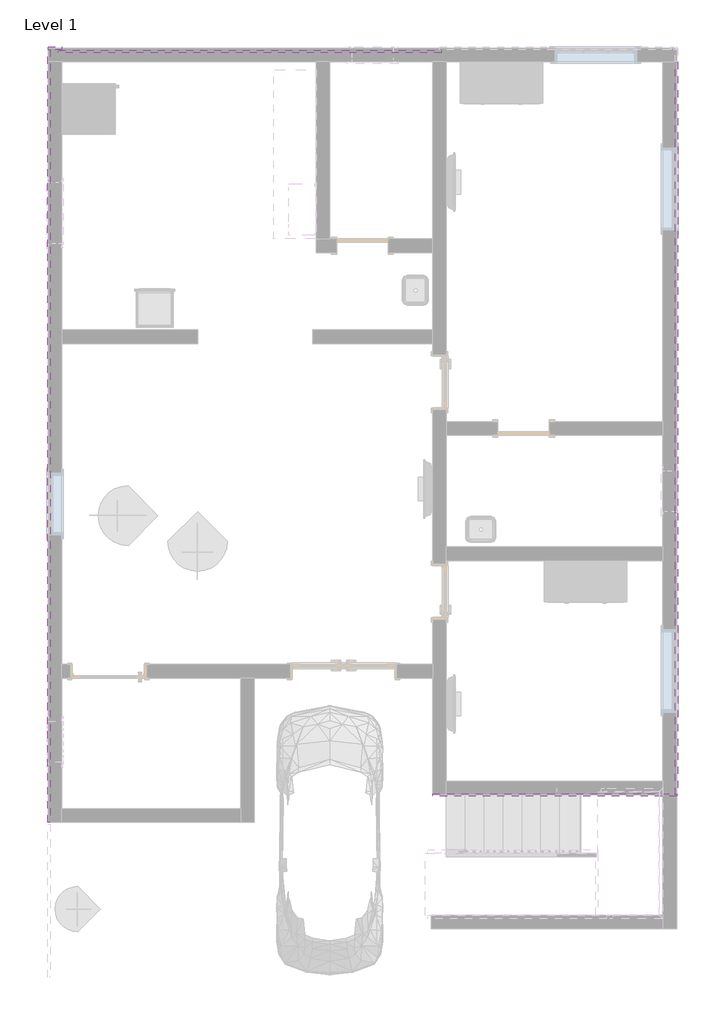
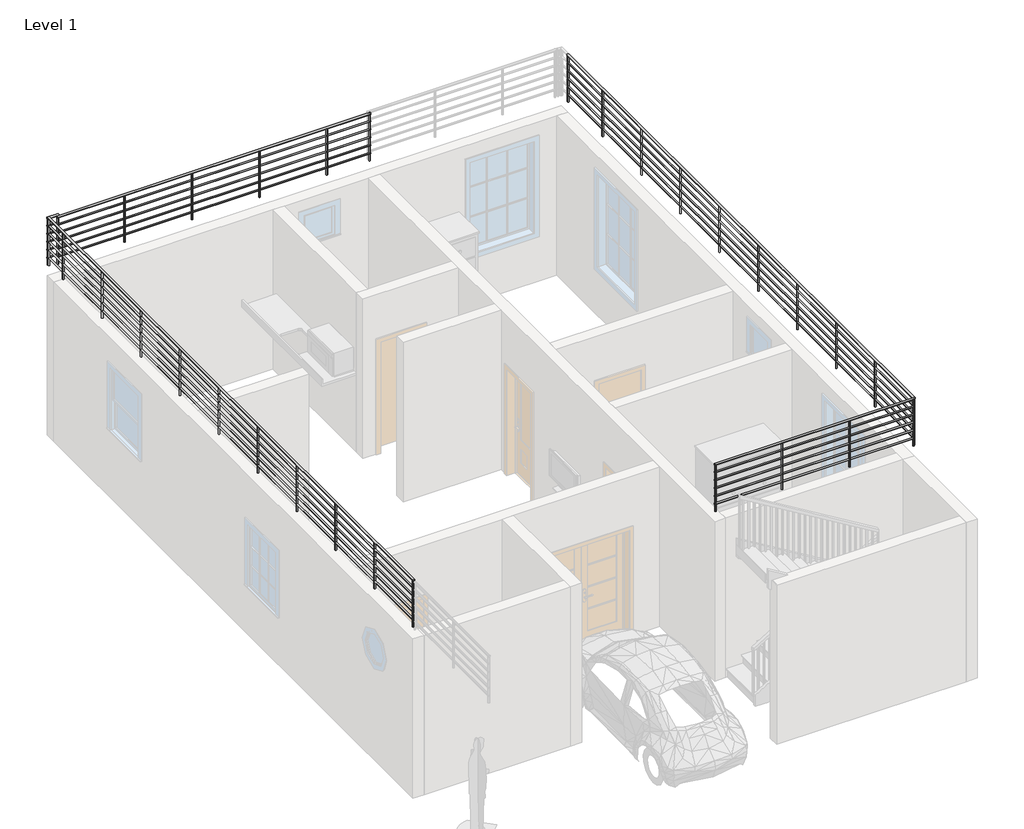
# One storey, part 3 of 4: 5 railings.
"""IFC4 building model written with IfcOpenShell, lengths in millimetres."""

from ifc_helpers import new_model, si_unit, point, frame, frame_2d, origin, place, context, project, spatial, circle_curve, trimmed, segment, composite_curve, outline, extrude, element, save

model = new_model("IFC4")

# Units and contexts
model_context = context("Model", 3, world=origin())
ifc_project = project(units=[si_unit("LENGTHUNIT", "METRE", prefix="MILLI")], contexts=[model_context])

# Site, building, storey
site = spatial("IfcSite", under=ifc_project)
building = spatial("IfcBuilding", under=site)
storey = spatial("IfcBuildingStorey", under=building, Name="Level 1", Elevation=0.0)

# Railings
placement = place(None, origin())
element("IfcRailing", 1, ObjectType="Handrail - Pipe", at=placement, inside=storey, context=model_context, shape_type="SweptSolid", body=[
    extrude(outline(composite_curve([segment(trimmed(circle_curve(frame_2d((4165.6002567, -14409.9389568)), 19.05), [point((4165.6002567, -14390.8889568))], [point((4165.6002567, -14428.9889568))], False, "CARTESIAN"), True, "CONTINUOUS"), segment(trimmed(circle_curve(frame_2d((4165.6002567, -14409.9389568)), 19.05), [point((4165.6002567, -14428.9889568))], [point((4165.6002567, -14390.8889568))], False, "CARTESIAN"), True, "CONTINUOUS")], self_intersect=False)), frame((0.0, 3652.9401605, 0.0), z_axis=(0.0, 1.0, 0.0), x_axis=(0.0, 0.0, 1.0)), (0.0, 0.0, 1.0), 11430.0),
    extrude(outline(composite_curve([segment(trimmed(circle_curve(frame_2d((4019.5502567, -14409.9389568)), 12.7), [point((4019.5502567, -14422.6389568))], [point((4019.5502567, -14397.2389568))], False, "CARTESIAN"), True, "CONTINUOUS"), segment(trimmed(circle_curve(frame_2d((4019.5502567, -14409.9389568)), 12.7), [point((4019.5502567, -14397.2389568))], [point((4019.5502567, -14422.6389568))], False, "CARTESIAN"), True, "CONTINUOUS")], self_intersect=False)), frame((0.0, 3652.9401605, 0.0), z_axis=(0.0, 1.0, 0.0), x_axis=(0.0, 0.0, 1.0)), (0.0, 0.0, 1.0), 11430.0),
    extrude(outline(composite_curve([segment(trimmed(circle_curve(frame_2d((3867.1502567, -14409.9389568)), 12.7), [point((3867.1502567, -14422.6389568))], [point((3867.1502567, -14397.2389568))], False, "CARTESIAN"), True, "CONTINUOUS"), segment(trimmed(circle_curve(frame_2d((3867.1502567, -14409.9389568)), 12.7), [point((3867.1502567, -14397.2389568))], [point((3867.1502567, -14422.6389568))], False, "CARTESIAN"), True, "CONTINUOUS")], self_intersect=False)), frame((0.0, 3652.9401605, 0.0), z_axis=(0.0, 1.0, 0.0), x_axis=(0.0, 0.0, 1.0)), (0.0, 0.0, 1.0), 11430.0),
    extrude(outline(composite_curve([segment(trimmed(circle_curve(frame_2d((3714.7502567, -14409.9389568)), 12.7), [point((3714.7502567, -14422.6389568))], [point((3714.7502567, -14397.2389568))], False, "CARTESIAN"), True, "CONTINUOUS"), segment(trimmed(circle_curve(frame_2d((3714.7502567, -14409.9389568)), 12.7), [point((3714.7502567, -14397.2389568))], [point((3714.7502567, -14422.6389568))], False, "CARTESIAN"), True, "CONTINUOUS")], self_intersect=False)), frame((0.0, 3652.9401605, 0.0), z_axis=(0.0, 1.0, 0.0), x_axis=(0.0, 0.0, 1.0)), (0.0, 0.0, 1.0), 11430.0),
    extrude(outline(composite_curve([segment(trimmed(circle_curve(frame_2d((3562.3502567, -14409.9389568)), 12.7), [point((3562.3502567, -14422.6389568))], [point((3562.3502567, -14397.2389568))], False, "CARTESIAN"), True, "CONTINUOUS"), segment(trimmed(circle_curve(frame_2d((3562.3502567, -14409.9389568)), 12.7), [point((3562.3502567, -14397.2389568))], [point((3562.3502567, -14422.6389568))], False, "CARTESIAN"), True, "CONTINUOUS")], self_intersect=False)), frame((0.0, 3652.9401605, 0.0), z_axis=(0.0, 1.0, 0.0), x_axis=(0.0, 0.0, 1.0)), (0.0, 0.0, 1.0), 11430.0),
    extrude(outline(composite_curve([segment(trimmed(circle_curve(frame_2d((3409.9502567, -14409.9389568)), 12.7), [point((3409.9502567, -14422.6389568))], [point((3409.9502567, -14397.2389568))], False, "CARTESIAN"), True, "CONTINUOUS"), segment(trimmed(circle_curve(frame_2d((3409.9502567, -14409.9389568)), 12.7), [point((3409.9502567, -14397.2389568))], [point((3409.9502567, -14422.6389568))], False, "CARTESIAN"), True, "CONTINUOUS")], self_intersect=False)), frame((0.0, 3652.9401605, 0.0), z_axis=(0.0, 1.0, 0.0), x_axis=(0.0, 0.0, 1.0)), (0.0, 0.0, 1.0), 11430.0),
    extrude(outline(composite_curve([segment(trimmed(circle_curve(frame_2d((-14409.9389568, 14625.7401605)), 12.7), [point((-14422.6389568, 14625.7401605))], [point((-14397.2389568, 14625.7401605))], False, "CARTESIAN"), True, "CONTINUOUS"), segment(trimmed(circle_curve(frame_2d((-14409.9389568, 14625.7401605)), 12.7), [point((-14397.2389568, 14625.7401605))], [point((-14422.6389568, 14625.7401605))], False, "CARTESIAN"), True, "CONTINUOUS")], self_intersect=False)), frame((0.0, 0.0, 3270.2502567), z_axis=(0.0, 0.0, 1.0), x_axis=(1.0, 0.0, 0.0)), (0.0, 0.0, 1.0), 876.3),
    extrude(outline(composite_curve([segment(trimmed(circle_curve(frame_2d((-14409.9389568, 13406.5401605)), 12.7), [point((-14422.6389568, 13406.5401605))], [point((-14397.2389568, 13406.5401605))], False, "CARTESIAN"), True, "CONTINUOUS"), segment(trimmed(circle_curve(frame_2d((-14409.9389568, 13406.5401605)), 12.7), [point((-14397.2389568, 13406.5401605))], [point((-14422.6389568, 13406.5401605))], False, "CARTESIAN"), True, "CONTINUOUS")], self_intersect=False)), frame((0.0, 0.0, 3270.2502567), z_axis=(0.0, 0.0, 1.0), x_axis=(1.0, 0.0, 0.0)), (0.0, 0.0, 1.0), 876.3),
    extrude(outline(composite_curve([segment(trimmed(circle_curve(frame_2d((-14409.9389568, 12187.3401605)), 12.7), [point((-14422.6389568, 12187.3401605))], [point((-14397.2389568, 12187.3401605))], False, "CARTESIAN"), True, "CONTINUOUS"), segment(trimmed(circle_curve(frame_2d((-14409.9389568, 12187.3401605)), 12.7), [point((-14397.2389568, 12187.3401605))], [point((-14422.6389568, 12187.3401605))], False, "CARTESIAN"), True, "CONTINUOUS")], self_intersect=False)), frame((0.0, 0.0, 3270.2502567), z_axis=(0.0, 0.0, 1.0), x_axis=(1.0, 0.0, 0.0)), (0.0, 0.0, 1.0), 876.3),
    extrude(outline(composite_curve([segment(trimmed(circle_curve(frame_2d((-14409.9389568, 10968.1401605)), 12.7), [point((-14422.6389568, 10968.1401605))], [point((-14397.2389568, 10968.1401605))], False, "CARTESIAN"), True, "CONTINUOUS"), segment(trimmed(circle_curve(frame_2d((-14409.9389568, 10968.1401605)), 12.7), [point((-14397.2389568, 10968.1401605))], [point((-14422.6389568, 10968.1401605))], False, "CARTESIAN"), True, "CONTINUOUS")], self_intersect=False)), frame((0.0, 0.0, 3270.2502567), z_axis=(0.0, 0.0, 1.0), x_axis=(1.0, 0.0, 0.0)), (0.0, 0.0, 1.0), 876.3),
    extrude(outline(composite_curve([segment(trimmed(circle_curve(frame_2d((-14409.9389568, 9748.9401605)), 12.7), [point((-14422.6389568, 9748.9401605))], [point((-14397.2389568, 9748.9401605))], False, "CARTESIAN"), True, "CONTINUOUS"), segment(trimmed(circle_curve(frame_2d((-14409.9389568, 9748.9401605)), 12.7), [point((-14397.2389568, 9748.9401605))], [point((-14422.6389568, 9748.9401605))], False, "CARTESIAN"), True, "CONTINUOUS")], self_intersect=False)), frame((0.0, 0.0, 3270.2502567), z_axis=(0.0, 0.0, 1.0), x_axis=(1.0, 0.0, 0.0)), (0.0, 0.0, 1.0), 876.3),
    extrude(outline(composite_curve([segment(trimmed(circle_curve(frame_2d((-14409.9389568, 8529.7401605)), 12.7), [point((-14422.6389568, 8529.7401605))], [point((-14397.2389568, 8529.7401605))], False, "CARTESIAN"), True, "CONTINUOUS"), segment(trimmed(circle_curve(frame_2d((-14409.9389568, 8529.7401605)), 12.7), [point((-14397.2389568, 8529.7401605))], [point((-14422.6389568, 8529.7401605))], False, "CARTESIAN"), True, "CONTINUOUS")], self_intersect=False)), frame((0.0, 0.0, 3270.2502567), z_axis=(0.0, 0.0, 1.0), x_axis=(1.0, 0.0, 0.0)), (0.0, 0.0, 1.0), 876.3),
    extrude(outline(composite_curve([segment(trimmed(circle_curve(frame_2d((-14409.9389568, 7310.5401605)), 12.7), [point((-14422.6389568, 7310.5401605))], [point((-14397.2389568, 7310.5401605))], False, "CARTESIAN"), True, "CONTINUOUS"), segment(trimmed(circle_curve(frame_2d((-14409.9389568, 7310.5401605)), 12.7), [point((-14397.2389568, 7310.5401605))], [point((-14422.6389568, 7310.5401605))], False, "CARTESIAN"), True, "CONTINUOUS")], self_intersect=False)), frame((0.0, 0.0, 3270.2502567), z_axis=(0.0, 0.0, 1.0), x_axis=(1.0, 0.0, 0.0)), (0.0, 0.0, 1.0), 876.3),
    extrude(outline(composite_curve([segment(trimmed(circle_curve(frame_2d((-14409.9389568, 6091.3401605)), 12.7), [point((-14422.6389568, 6091.3401605))], [point((-14397.2389568, 6091.3401605))], False, "CARTESIAN"), True, "CONTINUOUS"), segment(trimmed(circle_curve(frame_2d((-14409.9389568, 6091.3401605)), 12.7), [point((-14397.2389568, 6091.3401605))], [point((-14422.6389568, 6091.3401605))], False, "CARTESIAN"), True, "CONTINUOUS")], self_intersect=False)), frame((0.0, 0.0, 3270.2502567), z_axis=(0.0, 0.0, 1.0), x_axis=(1.0, 0.0, 0.0)), (0.0, 0.0, 1.0), 876.3),
    extrude(outline(composite_curve([segment(trimmed(circle_curve(frame_2d((-14409.9389568, 4872.1401605)), 12.7), [point((-14422.6389568, 4872.1401605))], [point((-14397.2389568, 4872.1401605))], False, "CARTESIAN"), True, "CONTINUOUS"), segment(trimmed(circle_curve(frame_2d((-14409.9389568, 4872.1401605)), 12.7), [point((-14397.2389568, 4872.1401605))], [point((-14422.6389568, 4872.1401605))], False, "CARTESIAN"), True, "CONTINUOUS")], self_intersect=False)), frame((0.0, 0.0, 3270.2502567), z_axis=(0.0, 0.0, 1.0), x_axis=(1.0, 0.0, 0.0)), (0.0, 0.0, 1.0), 876.3),
    extrude(outline(composite_curve([segment(trimmed(circle_curve(frame_2d((-14409.9389568, 15070.2401605)), 12.7), [point((-14422.6389568, 15070.2401605))], [point((-14397.2389568, 15070.2401605))], False, "CARTESIAN"), True, "CONTINUOUS"), segment(trimmed(circle_curve(frame_2d((-14409.9389568, 15070.2401605)), 12.7), [point((-14397.2389568, 15070.2401605))], [point((-14422.6389568, 15070.2401605))], False, "CARTESIAN"), True, "CONTINUOUS")], self_intersect=False)), frame((0.0, 0.0, 3270.2502567), z_axis=(0.0, 0.0, 1.0), x_axis=(1.0, 0.0, 0.0)), (0.0, 0.0, 1.0), 876.3),
    extrude(outline(composite_curve([segment(trimmed(circle_curve(frame_2d((-14409.9389568, 3665.6401605)), 12.7), [point((-14422.6389568, 3665.6401605))], [point((-14397.2389568, 3665.6401605))], False, "CARTESIAN"), True, "CONTINUOUS"), segment(trimmed(circle_curve(frame_2d((-14409.9389568, 3665.6401605)), 12.7), [point((-14397.2389568, 3665.6401605))], [point((-14422.6389568, 3665.6401605))], False, "CARTESIAN"), True, "CONTINUOUS")], self_intersect=False)), frame((0.0, 0.0, 3270.2502567), z_axis=(0.0, 0.0, 1.0), x_axis=(1.0, 0.0, 0.0)), (0.0, 0.0, 1.0), 876.3),
])
element("IfcRailing", 2, ObjectType="Handrail - Pipe", at=placement, inside=storey, context=model_context, shape_type="SweptSolid", body=[
    extrude(outline(composite_curve([segment(trimmed(circle_curve(frame_2d((15057.9844698, 4146.55)), 19.05), [point((15038.9344698, 4146.55))], [point((15077.0344698, 4146.55))], False, "CARTESIAN"), True, "CONTINUOUS"), segment(trimmed(circle_curve(frame_2d((15057.9844698, 4146.55)), 19.05), [point((15077.0344698, 4146.55))], [point((15038.9344698, 4146.55))], False, "CARTESIAN"), True, "CONTINUOUS")], self_intersect=False)), frame((-14272.3568408, 0.0, 0.0), z_axis=(1.0, 0.0, 0.0), x_axis=(0.0, 1.0, 0.0)), (0.0, 0.0, 1.0), 5664.2),
    extrude(outline(composite_curve([segment(trimmed(circle_curve(frame_2d((15057.9844698, 4000.5)), 12.7), [point((15070.6844698, 4000.5))], [point((15045.2844698, 4000.5))], False, "CARTESIAN"), True, "CONTINUOUS"), segment(trimmed(circle_curve(frame_2d((15057.9844698, 4000.5)), 12.7), [point((15045.2844698, 4000.5))], [point((15070.6844698, 4000.5))], False, "CARTESIAN"), True, "CONTINUOUS")], self_intersect=False)), frame((-14272.3568408, 0.0, 0.0), z_axis=(1.0, 0.0, 0.0), x_axis=(0.0, 1.0, 0.0)), (0.0, 0.0, 1.0), 5664.2),
    extrude(outline(composite_curve([segment(trimmed(circle_curve(frame_2d((15057.9844698, 3848.1)), 12.7), [point((15070.6844698, 3848.1))], [point((15045.2844698, 3848.1))], False, "CARTESIAN"), True, "CONTINUOUS"), segment(trimmed(circle_curve(frame_2d((15057.9844698, 3848.1)), 12.7), [point((15045.2844698, 3848.1))], [point((15070.6844698, 3848.1))], False, "CARTESIAN"), True, "CONTINUOUS")], self_intersect=False)), frame((-14272.3568408, 0.0, 0.0), z_axis=(1.0, 0.0, 0.0), x_axis=(0.0, 1.0, 0.0)), (0.0, 0.0, 1.0), 5664.2),
    extrude(outline(composite_curve([segment(trimmed(circle_curve(frame_2d((15057.9844698, 3695.7)), 12.7), [point((15070.6844698, 3695.7))], [point((15045.2844698, 3695.7))], False, "CARTESIAN"), True, "CONTINUOUS"), segment(trimmed(circle_curve(frame_2d((15057.9844698, 3695.7)), 12.7), [point((15045.2844698, 3695.7))], [point((15070.6844698, 3695.7))], False, "CARTESIAN"), True, "CONTINUOUS")], self_intersect=False)), frame((-14272.3568408, 0.0, 0.0), z_axis=(1.0, 0.0, 0.0), x_axis=(0.0, 1.0, 0.0)), (0.0, 0.0, 1.0), 5664.2),
    extrude(outline(composite_curve([segment(trimmed(circle_curve(frame_2d((15057.9844698, 3543.3)), 12.7), [point((15070.6844698, 3543.3))], [point((15045.2844698, 3543.3))], False, "CARTESIAN"), True, "CONTINUOUS"), segment(trimmed(circle_curve(frame_2d((15057.9844698, 3543.3)), 12.7), [point((15045.2844698, 3543.3))], [point((15070.6844698, 3543.3))], False, "CARTESIAN"), True, "CONTINUOUS")], self_intersect=False)), frame((-14272.3568408, 0.0, 0.0), z_axis=(1.0, 0.0, 0.0), x_axis=(0.0, 1.0, 0.0)), (0.0, 0.0, 1.0), 5664.2),
    extrude(outline(composite_curve([segment(trimmed(circle_curve(frame_2d((15057.9844698, 3390.9)), 12.7), [point((15070.6844698, 3390.9))], [point((15045.2844698, 3390.9))], False, "CARTESIAN"), True, "CONTINUOUS"), segment(trimmed(circle_curve(frame_2d((15057.9844698, 3390.9)), 12.7), [point((15045.2844698, 3390.9))], [point((15070.6844698, 3390.9))], False, "CARTESIAN"), True, "CONTINUOUS")], self_intersect=False)), frame((-14272.3568408, 0.0, 0.0), z_axis=(1.0, 0.0, 0.0), x_axis=(0.0, 1.0, 0.0)), (0.0, 0.0, 1.0), 5664.2),
    extrude(outline(composite_curve([segment(trimmed(circle_curve(frame_2d((-9395.5568408, 15057.9844698)), 12.7), [point((-9395.5568408, 15070.6844698))], [point((-9395.5568408, 15045.2844698))], False, "CARTESIAN"), True, "CONTINUOUS"), segment(trimmed(circle_curve(frame_2d((-9395.5568408, 15057.9844698)), 12.7), [point((-9395.5568408, 15045.2844698))], [point((-9395.5568408, 15070.6844698))], False, "CARTESIAN"), True, "CONTINUOUS")], self_intersect=False)), frame((0.0, 0.0, 3251.2), z_axis=(0.0, 0.0, 1.0), x_axis=(1.0, 0.0, 0.0)), (0.0, 0.0, 1.0), 876.3),
    extrude(outline(composite_curve([segment(trimmed(circle_curve(frame_2d((-10614.7568408, 15057.9844698)), 12.7), [point((-10614.7568408, 15070.6844698))], [point((-10614.7568408, 15045.2844698))], False, "CARTESIAN"), True, "CONTINUOUS"), segment(trimmed(circle_curve(frame_2d((-10614.7568408, 15057.9844698)), 12.7), [point((-10614.7568408, 15045.2844698))], [point((-10614.7568408, 15070.6844698))], False, "CARTESIAN"), True, "CONTINUOUS")], self_intersect=False)), frame((0.0, 0.0, 3251.2), z_axis=(0.0, 0.0, 1.0), x_axis=(1.0, 0.0, 0.0)), (0.0, 0.0, 1.0), 876.3),
    extrude(outline(composite_curve([segment(trimmed(circle_curve(frame_2d((-11833.9568408, 15057.9844698)), 12.7), [point((-11833.9568408, 15070.6844698))], [point((-11833.9568408, 15045.2844698))], False, "CARTESIAN"), True, "CONTINUOUS"), segment(trimmed(circle_curve(frame_2d((-11833.9568408, 15057.9844698)), 12.7), [point((-11833.9568408, 15045.2844698))], [point((-11833.9568408, 15070.6844698))], False, "CARTESIAN"), True, "CONTINUOUS")], self_intersect=False)), frame((0.0, 0.0, 3251.2), z_axis=(0.0, 0.0, 1.0), x_axis=(1.0, 0.0, 0.0)), (0.0, 0.0, 1.0), 876.3),
    extrude(outline(composite_curve([segment(trimmed(circle_curve(frame_2d((-13053.1568408, 15057.9844698)), 12.7), [point((-13053.1568408, 15070.6844698))], [point((-13053.1568408, 15045.2844698))], False, "CARTESIAN"), True, "CONTINUOUS"), segment(trimmed(circle_curve(frame_2d((-13053.1568408, 15057.9844698)), 12.7), [point((-13053.1568408, 15045.2844698))], [point((-13053.1568408, 15070.6844698))], False, "CARTESIAN"), True, "CONTINUOUS")], self_intersect=False)), frame((0.0, 0.0, 3251.2), z_axis=(0.0, 0.0, 1.0), x_axis=(1.0, 0.0, 0.0)), (0.0, 0.0, 1.0), 876.3),
    extrude(outline(composite_curve([segment(trimmed(circle_curve(frame_2d((-8620.8568408, 15057.9844698)), 12.7), [point((-8620.8568408, 15070.6844698))], [point((-8620.8568408, 15045.2844698))], False, "CARTESIAN"), True, "CONTINUOUS"), segment(trimmed(circle_curve(frame_2d((-8620.8568408, 15057.9844698)), 12.7), [point((-8620.8568408, 15045.2844698))], [point((-8620.8568408, 15070.6844698))], False, "CARTESIAN"), True, "CONTINUOUS")], self_intersect=False)), frame((0.0, 0.0, 3251.2), z_axis=(0.0, 0.0, 1.0), x_axis=(1.0, 0.0, 0.0)), (0.0, 0.0, 1.0), 876.3),
    extrude(outline(composite_curve([segment(trimmed(circle_curve(frame_2d((-14259.6568408, 15057.9844698)), 12.7), [point((-14259.6568408, 15070.6844698))], [point((-14259.6568408, 15045.2844698))], False, "CARTESIAN"), True, "CONTINUOUS"), segment(trimmed(circle_curve(frame_2d((-14259.6568408, 15057.9844698)), 12.7), [point((-14259.6568408, 15045.2844698))], [point((-14259.6568408, 15070.6844698))], False, "CARTESIAN"), True, "CONTINUOUS")], self_intersect=False)), frame((0.0, 0.0, 3251.2), z_axis=(0.0, 0.0, 1.0), x_axis=(1.0, 0.0, 0.0)), (0.0, 0.0, 1.0), 876.3),
])
element("IfcRailing", 3, ObjectType="Handrail - Pipe", at=placement, inside=storey, context=model_context, shape_type="SweptSolid", body=[
    extrude(outline(composite_curve([segment(trimmed(circle_curve(frame_2d((4059.1342758, 4146.55)), 19.05), [point((4040.0842758, 4146.55))], [point((4078.1842758, 4146.55))], False, "CARTESIAN"), True, "CONTINUOUS"), segment(trimmed(circle_curve(frame_2d((4059.1342758, 4146.55)), 19.05), [point((4078.1842758, 4146.55))], [point((4040.0842758, 4146.55))], False, "CARTESIAN"), True, "CONTINUOUS")], self_intersect=False)), frame((-8733.0389568, 0.0, 0.0), z_axis=(1.0, 0.0, 0.0), x_axis=(0.0, 1.0, 0.0)), (0.0, 0.0, 1.0), 3606.8),
    extrude(outline(composite_curve([segment(trimmed(circle_curve(frame_2d((4059.1342758, 4000.5)), 12.7), [point((4071.8342758, 4000.5))], [point((4046.4342758, 4000.5))], False, "CARTESIAN"), True, "CONTINUOUS"), segment(trimmed(circle_curve(frame_2d((4059.1342758, 4000.5)), 12.7), [point((4046.4342758, 4000.5))], [point((4071.8342758, 4000.5))], False, "CARTESIAN"), True, "CONTINUOUS")], self_intersect=False)), frame((-8733.0389568, 0.0, 0.0), z_axis=(1.0, 0.0, 0.0), x_axis=(0.0, 1.0, 0.0)), (0.0, 0.0, 1.0), 3606.8),
    extrude(outline(composite_curve([segment(trimmed(circle_curve(frame_2d((4059.1342758, 3848.1)), 12.7), [point((4071.8342758, 3848.1))], [point((4046.4342758, 3848.1))], False, "CARTESIAN"), True, "CONTINUOUS"), segment(trimmed(circle_curve(frame_2d((4059.1342758, 3848.1)), 12.7), [point((4046.4342758, 3848.1))], [point((4071.8342758, 3848.1))], False, "CARTESIAN"), True, "CONTINUOUS")], self_intersect=False)), frame((-8733.0389568, 0.0, 0.0), z_axis=(1.0, 0.0, 0.0), x_axis=(0.0, 1.0, 0.0)), (0.0, 0.0, 1.0), 3606.8),
    extrude(outline(composite_curve([segment(trimmed(circle_curve(frame_2d((4059.1342758, 3695.7)), 12.7), [point((4071.8342758, 3695.7))], [point((4046.4342758, 3695.7))], False, "CARTESIAN"), True, "CONTINUOUS"), segment(trimmed(circle_curve(frame_2d((4059.1342758, 3695.7)), 12.7), [point((4046.4342758, 3695.7))], [point((4071.8342758, 3695.7))], False, "CARTESIAN"), True, "CONTINUOUS")], self_intersect=False)), frame((-8733.0389568, 0.0, 0.0), z_axis=(1.0, 0.0, 0.0), x_axis=(0.0, 1.0, 0.0)), (0.0, 0.0, 1.0), 3606.8),
    extrude(outline(composite_curve([segment(trimmed(circle_curve(frame_2d((4059.1342758, 3543.3)), 12.7), [point((4071.8342758, 3543.3))], [point((4046.4342758, 3543.3))], False, "CARTESIAN"), True, "CONTINUOUS"), segment(trimmed(circle_curve(frame_2d((4059.1342758, 3543.3)), 12.7), [point((4046.4342758, 3543.3))], [point((4071.8342758, 3543.3))], False, "CARTESIAN"), True, "CONTINUOUS")], self_intersect=False)), frame((-8733.0389568, 0.0, 0.0), z_axis=(1.0, 0.0, 0.0), x_axis=(0.0, 1.0, 0.0)), (0.0, 0.0, 1.0), 3606.8),
    extrude(outline(composite_curve([segment(trimmed(circle_curve(frame_2d((4059.1342758, 3390.9)), 12.7), [point((4071.8342758, 3390.9))], [point((4046.4342758, 3390.9))], False, "CARTESIAN"), True, "CONTINUOUS"), segment(trimmed(circle_curve(frame_2d((4059.1342758, 3390.9)), 12.7), [point((4046.4342758, 3390.9))], [point((4071.8342758, 3390.9))], False, "CARTESIAN"), True, "CONTINUOUS")], self_intersect=False)), frame((-8733.0389568, 0.0, 0.0), z_axis=(1.0, 0.0, 0.0), x_axis=(0.0, 1.0, 0.0)), (0.0, 0.0, 1.0), 3606.8),
    extrude(outline(composite_curve([segment(trimmed(circle_curve(frame_2d((-6294.6389568, 4059.1342758)), 12.7), [point((-6294.6389568, 4071.8342758))], [point((-6294.6389568, 4046.4342758))], False, "CARTESIAN"), True, "CONTINUOUS"), segment(trimmed(circle_curve(frame_2d((-6294.6389568, 4059.1342758)), 12.7), [point((-6294.6389568, 4046.4342758))], [point((-6294.6389568, 4071.8342758))], False, "CARTESIAN"), True, "CONTINUOUS")], self_intersect=False)), frame((0.0, 0.0, 3251.2), z_axis=(0.0, 0.0, 1.0), x_axis=(1.0, 0.0, 0.0)), (0.0, 0.0, 1.0), 876.3),
    extrude(outline(composite_curve([segment(trimmed(circle_curve(frame_2d((-7513.8389568, 4059.1342758)), 12.7), [point((-7513.8389568, 4071.8342758))], [point((-7513.8389568, 4046.4342758))], False, "CARTESIAN"), True, "CONTINUOUS"), segment(trimmed(circle_curve(frame_2d((-7513.8389568, 4059.1342758)), 12.7), [point((-7513.8389568, 4046.4342758))], [point((-7513.8389568, 4071.8342758))], False, "CARTESIAN"), True, "CONTINUOUS")], self_intersect=False)), frame((0.0, 0.0, 3251.2), z_axis=(0.0, 0.0, 1.0), x_axis=(1.0, 0.0, 0.0)), (0.0, 0.0, 1.0), 876.3),
    extrude(outline(composite_curve([segment(trimmed(circle_curve(frame_2d((-5138.9389568, 4059.1342758)), 12.7), [point((-5138.9389568, 4071.8342758))], [point((-5138.9389568, 4046.4342758))], False, "CARTESIAN"), True, "CONTINUOUS"), segment(trimmed(circle_curve(frame_2d((-5138.9389568, 4059.1342758)), 12.7), [point((-5138.9389568, 4046.4342758))], [point((-5138.9389568, 4071.8342758))], False, "CARTESIAN"), True, "CONTINUOUS")], self_intersect=False)), frame((0.0, 0.0, 3251.2), z_axis=(0.0, 0.0, 1.0), x_axis=(1.0, 0.0, 0.0)), (0.0, 0.0, 1.0), 876.3),
    extrude(outline(composite_curve([segment(trimmed(circle_curve(frame_2d((-8720.3389568, 4059.1342758)), 12.7), [point((-8720.3389568, 4071.8342758))], [point((-8720.3389568, 4046.4342758))], False, "CARTESIAN"), True, "CONTINUOUS"), segment(trimmed(circle_curve(frame_2d((-8720.3389568, 4059.1342758)), 12.7), [point((-8720.3389568, 4046.4342758))], [point((-8720.3389568, 4071.8342758))], False, "CARTESIAN"), True, "CONTINUOUS")], self_intersect=False)), frame((0.0, 0.0, 3251.2), z_axis=(0.0, 0.0, 1.0), x_axis=(1.0, 0.0, 0.0)), (0.0, 0.0, 1.0), 876.3),
])
element("IfcRailing", 4, ObjectType="Handrail - Pipe", at=placement, inside=storey, context=model_context, shape_type="SweptSolid", body=[
    extrude(outline(composite_curve([segment(trimmed(circle_curve(frame_2d((4146.55, -5126.2389568)), 19.05), [point((4146.55, -5107.1889568))], [point((4146.55, -5145.2889568))], False, "CARTESIAN"), True, "CONTINUOUS"), segment(trimmed(circle_curve(frame_2d((4146.55, -5126.2389568)), 19.05), [point((4146.55, -5145.2889568))], [point((4146.55, -5107.1889568))], False, "CARTESIAN"), True, "CONTINUOUS")], self_intersect=False)), frame((0.0, 4059.1342758, 0.0), z_axis=(0.0, 1.0, 0.0), x_axis=(0.0, 0.0, 1.0)), (0.0, 0.0, 1.0), 10845.8),
    extrude(outline(composite_curve([segment(trimmed(circle_curve(frame_2d((4000.5, -5126.2389568)), 12.7), [point((4000.5, -5138.9389568))], [point((4000.5, -5113.5389568))], False, "CARTESIAN"), True, "CONTINUOUS"), segment(trimmed(circle_curve(frame_2d((4000.5, -5126.2389568)), 12.7), [point((4000.5, -5113.5389568))], [point((4000.5, -5138.9389568))], False, "CARTESIAN"), True, "CONTINUOUS")], self_intersect=False)), frame((0.0, 4059.1342758, 0.0), z_axis=(0.0, 1.0, 0.0), x_axis=(0.0, 0.0, 1.0)), (0.0, 0.0, 1.0), 10845.8),
    extrude(outline(composite_curve([segment(trimmed(circle_curve(frame_2d((3848.1, -5126.2389568)), 12.7), [point((3848.1, -5138.9389568))], [point((3848.1, -5113.5389568))], False, "CARTESIAN"), True, "CONTINUOUS"), segment(trimmed(circle_curve(frame_2d((3848.1, -5126.2389568)), 12.7), [point((3848.1, -5113.5389568))], [point((3848.1, -5138.9389568))], False, "CARTESIAN"), True, "CONTINUOUS")], self_intersect=False)), frame((0.0, 4059.1342758, 0.0), z_axis=(0.0, 1.0, 0.0), x_axis=(0.0, 0.0, 1.0)), (0.0, 0.0, 1.0), 10845.8),
    extrude(outline(composite_curve([segment(trimmed(circle_curve(frame_2d((3695.7, -5126.2389568)), 12.7), [point((3695.7, -5138.9389568))], [point((3695.7, -5113.5389568))], False, "CARTESIAN"), True, "CONTINUOUS"), segment(trimmed(circle_curve(frame_2d((3695.7, -5126.2389568)), 12.7), [point((3695.7, -5113.5389568))], [point((3695.7, -5138.9389568))], False, "CARTESIAN"), True, "CONTINUOUS")], self_intersect=False)), frame((0.0, 4059.1342758, 0.0), z_axis=(0.0, 1.0, 0.0), x_axis=(0.0, 0.0, 1.0)), (0.0, 0.0, 1.0), 10845.8),
    extrude(outline(composite_curve([segment(trimmed(circle_curve(frame_2d((3543.3, -5126.2389568)), 12.7), [point((3543.3, -5138.9389568))], [point((3543.3, -5113.5389568))], False, "CARTESIAN"), True, "CONTINUOUS"), segment(trimmed(circle_curve(frame_2d((3543.3, -5126.2389568)), 12.7), [point((3543.3, -5113.5389568))], [point((3543.3, -5138.9389568))], False, "CARTESIAN"), True, "CONTINUOUS")], self_intersect=False)), frame((0.0, 4059.1342758, 0.0), z_axis=(0.0, 1.0, 0.0), x_axis=(0.0, 0.0, 1.0)), (0.0, 0.0, 1.0), 10845.8),
    extrude(outline(composite_curve([segment(trimmed(circle_curve(frame_2d((3390.9, -5126.2389568)), 12.7), [point((3390.9, -5138.9389568))], [point((3390.9, -5113.5389568))], False, "CARTESIAN"), True, "CONTINUOUS"), segment(trimmed(circle_curve(frame_2d((3390.9, -5126.2389568)), 12.7), [point((3390.9, -5113.5389568))], [point((3390.9, -5138.9389568))], False, "CARTESIAN"), True, "CONTINUOUS")], self_intersect=False)), frame((0.0, 4059.1342758, 0.0), z_axis=(0.0, 1.0, 0.0), x_axis=(0.0, 0.0, 1.0)), (0.0, 0.0, 1.0), 10845.8),
    extrude(outline(composite_curve([segment(trimmed(circle_curve(frame_2d((-5126.2389568, 13812.7342758)), 12.7), [point((-5138.9389568, 13812.7342758))], [point((-5113.5389568, 13812.7342758))], False, "CARTESIAN"), True, "CONTINUOUS"), segment(trimmed(circle_curve(frame_2d((-5126.2389568, 13812.7342758)), 12.7), [point((-5113.5389568, 13812.7342758))], [point((-5138.9389568, 13812.7342758))], False, "CARTESIAN"), True, "CONTINUOUS")], self_intersect=False)), frame((0.0, 0.0, 3251.2), z_axis=(0.0, 0.0, 1.0), x_axis=(1.0, 0.0, 0.0)), (0.0, 0.0, 1.0), 876.3),
    extrude(outline(composite_curve([segment(trimmed(circle_curve(frame_2d((-5126.2389568, 12593.5342758)), 12.7), [point((-5138.9389568, 12593.5342758))], [point((-5113.5389568, 12593.5342758))], False, "CARTESIAN"), True, "CONTINUOUS"), segment(trimmed(circle_curve(frame_2d((-5126.2389568, 12593.5342758)), 12.7), [point((-5113.5389568, 12593.5342758))], [point((-5138.9389568, 12593.5342758))], False, "CARTESIAN"), True, "CONTINUOUS")], self_intersect=False)), frame((0.0, 0.0, 3251.2), z_axis=(0.0, 0.0, 1.0), x_axis=(1.0, 0.0, 0.0)), (0.0, 0.0, 1.0), 876.3),
    extrude(outline(composite_curve([segment(trimmed(circle_curve(frame_2d((-5126.2389568, 11374.3342758)), 12.7), [point((-5138.9389568, 11374.3342758))], [point((-5113.5389568, 11374.3342758))], False, "CARTESIAN"), True, "CONTINUOUS"), segment(trimmed(circle_curve(frame_2d((-5126.2389568, 11374.3342758)), 12.7), [point((-5113.5389568, 11374.3342758))], [point((-5138.9389568, 11374.3342758))], False, "CARTESIAN"), True, "CONTINUOUS")], self_intersect=False)), frame((0.0, 0.0, 3251.2), z_axis=(0.0, 0.0, 1.0), x_axis=(1.0, 0.0, 0.0)), (0.0, 0.0, 1.0), 876.3),
    extrude(outline(composite_curve([segment(trimmed(circle_curve(frame_2d((-5126.2389568, 10155.1342758)), 12.7), [point((-5138.9389568, 10155.1342758))], [point((-5113.5389568, 10155.1342758))], False, "CARTESIAN"), True, "CONTINUOUS"), segment(trimmed(circle_curve(frame_2d((-5126.2389568, 10155.1342758)), 12.7), [point((-5113.5389568, 10155.1342758))], [point((-5138.9389568, 10155.1342758))], False, "CARTESIAN"), True, "CONTINUOUS")], self_intersect=False)), frame((0.0, 0.0, 3251.2), z_axis=(0.0, 0.0, 1.0), x_axis=(1.0, 0.0, 0.0)), (0.0, 0.0, 1.0), 876.3),
    extrude(outline(composite_curve([segment(trimmed(circle_curve(frame_2d((-5126.2389568, 8935.9342758)), 12.7), [point((-5138.9389568, 8935.9342758))], [point((-5113.5389568, 8935.9342758))], False, "CARTESIAN"), True, "CONTINUOUS"), segment(trimmed(circle_curve(frame_2d((-5126.2389568, 8935.9342758)), 12.7), [point((-5113.5389568, 8935.9342758))], [point((-5138.9389568, 8935.9342758))], False, "CARTESIAN"), True, "CONTINUOUS")], self_intersect=False)), frame((0.0, 0.0, 3251.2), z_axis=(0.0, 0.0, 1.0), x_axis=(1.0, 0.0, 0.0)), (0.0, 0.0, 1.0), 876.3),
    extrude(outline(composite_curve([segment(trimmed(circle_curve(frame_2d((-5126.2389568, 7716.7342758)), 12.7), [point((-5138.9389568, 7716.7342758))], [point((-5113.5389568, 7716.7342758))], False, "CARTESIAN"), True, "CONTINUOUS"), segment(trimmed(circle_curve(frame_2d((-5126.2389568, 7716.7342758)), 12.7), [point((-5113.5389568, 7716.7342758))], [point((-5138.9389568, 7716.7342758))], False, "CARTESIAN"), True, "CONTINUOUS")], self_intersect=False)), frame((0.0, 0.0, 3251.2), z_axis=(0.0, 0.0, 1.0), x_axis=(1.0, 0.0, 0.0)), (0.0, 0.0, 1.0), 876.3),
    extrude(outline(composite_curve([segment(trimmed(circle_curve(frame_2d((-5126.2389568, 6497.5342758)), 12.7), [point((-5138.9389568, 6497.5342758))], [point((-5113.5389568, 6497.5342758))], False, "CARTESIAN"), True, "CONTINUOUS"), segment(trimmed(circle_curve(frame_2d((-5126.2389568, 6497.5342758)), 12.7), [point((-5113.5389568, 6497.5342758))], [point((-5138.9389568, 6497.5342758))], False, "CARTESIAN"), True, "CONTINUOUS")], self_intersect=False)), frame((0.0, 0.0, 3251.2), z_axis=(0.0, 0.0, 1.0), x_axis=(1.0, 0.0, 0.0)), (0.0, 0.0, 1.0), 876.3),
    extrude(outline(composite_curve([segment(trimmed(circle_curve(frame_2d((-5126.2389568, 5278.3342758)), 12.7), [point((-5138.9389568, 5278.3342758))], [point((-5113.5389568, 5278.3342758))], False, "CARTESIAN"), True, "CONTINUOUS"), segment(trimmed(circle_curve(frame_2d((-5126.2389568, 5278.3342758)), 12.7), [point((-5113.5389568, 5278.3342758))], [point((-5138.9389568, 5278.3342758))], False, "CARTESIAN"), True, "CONTINUOUS")], self_intersect=False)), frame((0.0, 0.0, 3251.2), z_axis=(0.0, 0.0, 1.0), x_axis=(1.0, 0.0, 0.0)), (0.0, 0.0, 1.0), 876.3),
    extrude(outline(composite_curve([segment(trimmed(circle_curve(frame_2d((-5126.2389568, 14892.2342758)), 12.7), [point((-5138.9389568, 14892.2342758))], [point((-5113.5389568, 14892.2342758))], False, "CARTESIAN"), True, "CONTINUOUS"), segment(trimmed(circle_curve(frame_2d((-5126.2389568, 14892.2342758)), 12.7), [point((-5113.5389568, 14892.2342758))], [point((-5138.9389568, 14892.2342758))], False, "CARTESIAN"), True, "CONTINUOUS")], self_intersect=False)), frame((0.0, 0.0, 3251.2), z_axis=(0.0, 0.0, 1.0), x_axis=(1.0, 0.0, 0.0)), (0.0, 0.0, 1.0), 876.3),
    extrude(outline(composite_curve([segment(trimmed(circle_curve(frame_2d((-5126.2389568, 4071.8342758)), 12.7), [point((-5138.9389568, 4071.8342758))], [point((-5113.5389568, 4071.8342758))], False, "CARTESIAN"), True, "CONTINUOUS"), segment(trimmed(circle_curve(frame_2d((-5126.2389568, 4071.8342758)), 12.7), [point((-5113.5389568, 4071.8342758))], [point((-5138.9389568, 4071.8342758))], False, "CARTESIAN"), True, "CONTINUOUS")], self_intersect=False)), frame((0.0, 0.0, 3251.2), z_axis=(0.0, 0.0, 1.0), x_axis=(1.0, 0.0, 0.0)), (0.0, 0.0, 1.0), 876.3),
])
element("IfcRailing", 5, ObjectType="Handrail - Pipe", at=placement, inside=storey, context=model_context, shape_type="SweptSolid", body=[
    extrude(outline(composite_curve([segment(trimmed(circle_curve(frame_2d((15108.1342758, 4146.55)), 19.05), [point((15089.0842758, 4146.55))], [point((15127.1842758, 4146.55))], False, "CARTESIAN"), True, "CONTINUOUS"), segment(trimmed(circle_curve(frame_2d((15108.1342758, 4146.55)), 19.05), [point((15127.1842758, 4146.55))], [point((15089.0842758, 4146.55))], False, "CARTESIAN"), True, "CONTINUOUS")], self_intersect=False)), frame((-14422.6389568, 0.0, 0.0), z_axis=(1.0, 0.0, 0.0), x_axis=(0.0, 1.0, 0.0)), (0.0, 0.0, 1.0), 203.2),
    extrude(outline(composite_curve([segment(trimmed(circle_curve(frame_2d((15108.1342758, 4000.5)), 12.7), [point((15120.8342758, 4000.5))], [point((15095.4342758, 4000.5))], False, "CARTESIAN"), True, "CONTINUOUS"), segment(trimmed(circle_curve(frame_2d((15108.1342758, 4000.5)), 12.7), [point((15095.4342758, 4000.5))], [point((15120.8342758, 4000.5))], False, "CARTESIAN"), True, "CONTINUOUS")], self_intersect=False)), frame((-14422.6389568, 0.0, 0.0), z_axis=(1.0, 0.0, 0.0), x_axis=(0.0, 1.0, 0.0)), (0.0, 0.0, 1.0), 203.2),
    extrude(outline(composite_curve([segment(trimmed(circle_curve(frame_2d((15108.1342758, 3848.1)), 12.7), [point((15120.8342758, 3848.1))], [point((15095.4342758, 3848.1))], False, "CARTESIAN"), True, "CONTINUOUS"), segment(trimmed(circle_curve(frame_2d((15108.1342758, 3848.1)), 12.7), [point((15095.4342758, 3848.1))], [point((15120.8342758, 3848.1))], False, "CARTESIAN"), True, "CONTINUOUS")], self_intersect=False)), frame((-14422.6389568, 0.0, 0.0), z_axis=(1.0, 0.0, 0.0), x_axis=(0.0, 1.0, 0.0)), (0.0, 0.0, 1.0), 203.2),
    extrude(outline(composite_curve([segment(trimmed(circle_curve(frame_2d((15108.1342758, 3695.7)), 12.7), [point((15120.8342758, 3695.7))], [point((15095.4342758, 3695.7))], False, "CARTESIAN"), True, "CONTINUOUS"), segment(trimmed(circle_curve(frame_2d((15108.1342758, 3695.7)), 12.7), [point((15095.4342758, 3695.7))], [point((15120.8342758, 3695.7))], False, "CARTESIAN"), True, "CONTINUOUS")], self_intersect=False)), frame((-14422.6389568, 0.0, 0.0), z_axis=(1.0, 0.0, 0.0), x_axis=(0.0, 1.0, 0.0)), (0.0, 0.0, 1.0), 203.2),
    extrude(outline(composite_curve([segment(trimmed(circle_curve(frame_2d((15108.1342758, 3543.3)), 12.7), [point((15120.8342758, 3543.3))], [point((15095.4342758, 3543.3))], False, "CARTESIAN"), True, "CONTINUOUS"), segment(trimmed(circle_curve(frame_2d((15108.1342758, 3543.3)), 12.7), [point((15095.4342758, 3543.3))], [point((15120.8342758, 3543.3))], False, "CARTESIAN"), True, "CONTINUOUS")], self_intersect=False)), frame((-14422.6389568, 0.0, 0.0), z_axis=(1.0, 0.0, 0.0), x_axis=(0.0, 1.0, 0.0)), (0.0, 0.0, 1.0), 203.2),
    extrude(outline(composite_curve([segment(trimmed(circle_curve(frame_2d((15108.1342758, 3390.9)), 12.7), [point((15120.8342758, 3390.9))], [point((15095.4342758, 3390.9))], False, "CARTESIAN"), True, "CONTINUOUS"), segment(trimmed(circle_curve(frame_2d((15108.1342758, 3390.9)), 12.7), [point((15095.4342758, 3390.9))], [point((15120.8342758, 3390.9))], False, "CARTESIAN"), True, "CONTINUOUS")], self_intersect=False)), frame((-14422.6389568, 0.0, 0.0), z_axis=(1.0, 0.0, 0.0), x_axis=(0.0, 1.0, 0.0)), (0.0, 0.0, 1.0), 203.2),
    extrude(outline(composite_curve([segment(trimmed(circle_curve(frame_2d((-14232.1389568, 15108.1342758)), 12.7), [point((-14232.1389568, 15120.8342758))], [point((-14232.1389568, 15095.4342758))], False, "CARTESIAN"), True, "CONTINUOUS"), segment(trimmed(circle_curve(frame_2d((-14232.1389568, 15108.1342758)), 12.7), [point((-14232.1389568, 15095.4342758))], [point((-14232.1389568, 15120.8342758))], False, "CARTESIAN"), True, "CONTINUOUS")], self_intersect=False)), frame((0.0, 0.0, 3251.2), z_axis=(0.0, 0.0, 1.0), x_axis=(1.0, 0.0, 0.0)), (0.0, 0.0, 1.0), 876.3),
    extrude(outline(composite_curve([segment(trimmed(circle_curve(frame_2d((-14409.9389568, 15108.1342758)), 12.7), [point((-14409.9389568, 15120.8342758))], [point((-14409.9389568, 15095.4342758))], False, "CARTESIAN"), True, "CONTINUOUS"), segment(trimmed(circle_curve(frame_2d((-14409.9389568, 15108.1342758)), 12.7), [point((-14409.9389568, 15095.4342758))], [point((-14409.9389568, 15120.8342758))], False, "CARTESIAN"), True, "CONTINUOUS")], self_intersect=False)), frame((0.0, 0.0, 3251.2), z_axis=(0.0, 0.0, 1.0), x_axis=(1.0, 0.0, 0.0)), (0.0, 0.0, 1.0), 876.3),
])

save(model, "model.ifc")

# Revit data of these elements
# Type "Handrail - Pipe"
#   Assembly Code = "C2010400"
#   built-in parameter 1008612 = 0.0416667 (stored number, unit not read)
#   built-in parameter 1008611 = 0.0833333 (stored number, unit not read)
#   built-in parameter 1008609 = 4 (stored number, unit not read)
#   built-in parameter 1008604 = 0.166667 (stored number, unit not read)
#   built-in parameter 1008603 = 0.166667 (stored number, unit not read)
#   Railing Height = 3' - 0"
#   built-in parameter 1008630 = 2
#   built-in parameter 1008610 = 1
#   built-in parameter 1008605 = 1
#   built-in parameter 1008618 = Baluster - Round : 1"
# Element 1 (IfcRailing, "Handrail - Pipe")
#   built-in parameter 1008621 = 10.7292 (stored number, unit not read)
#   Phase Created = New Construction
# Elements 2, 3, 4, 5 (IfcRailing, "Handrail - Pipe")
#   built-in parameter 1008621 = 10.6667 (stored number, unit not read)
#   Phase Created = New Construction
